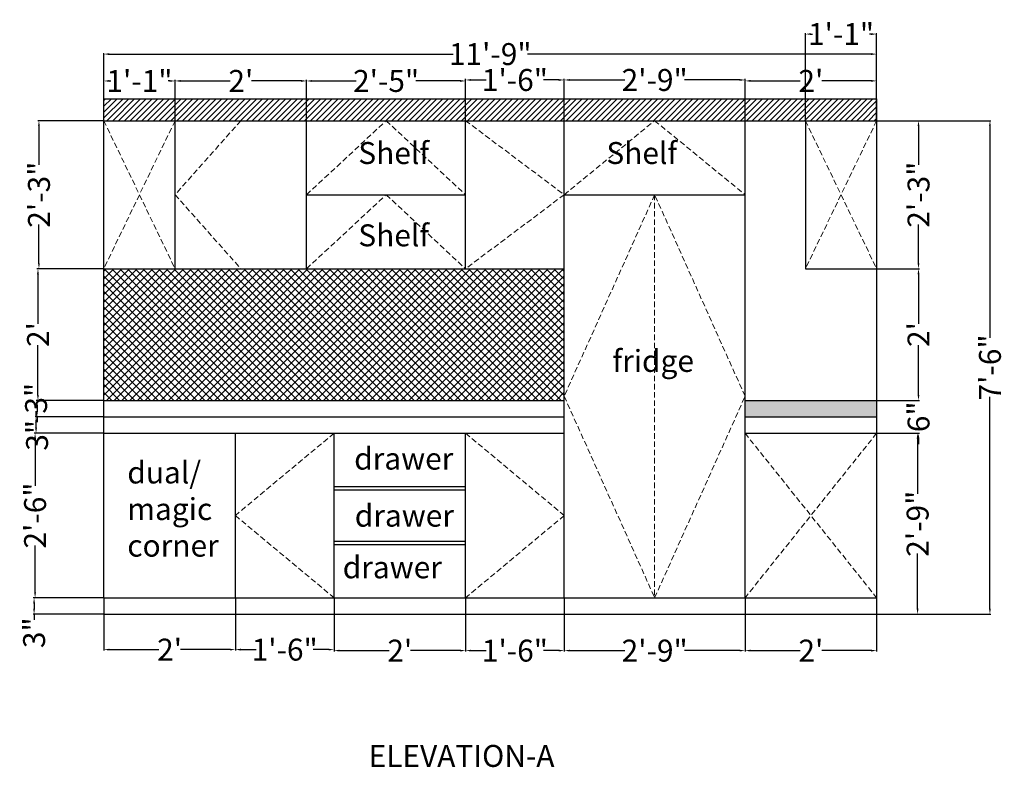
# Model space of a CAD drawing. Units: inches. Extents: x 560 to 756, y 301 to 635.
# Tile 1 of 2: x 560 to 740, y 301 to 437. Entities that reach past the tile are written whole.
import ezdxf

# ---------------------------------------------------------------- set-up
doc = ezdxf.new("R2010")
doc.units = ezdxf.units.IN
doc.header["$LTSCALE"] = 2
doc.header["$MEASUREMENT"] = 0
doc.linetypes.add('DASHED', pattern=[0.75, 0.5, -0.25])
for name, color, linetype, lineweight in [('A-ANNO-DIMS', 2, 'Continuous', 18), ('A-ANNO-TEXT', 3, 'Continuous', 18), ('A-ELEV', 7, 'Continuous', 25), ('A-ELEV-OPEN', 8, 'DASHED', 13), ('A-ELEV-PATT', 250, 'Continuous', 13)]:
    doc.layers.add(name, color=color, linetype=linetype, lineweight=lineweight)
doc.styles.get("Standard").update_dxf_attribs({"font": 'arial.ttf'})
doc.dimstyles.get("Standard").update_dxf_attribs({"dimtxt": 4, "dimasz": 1, "dimexe": 0.18, "dimexo": 0.0625, "dimgap": 0.09, "dimtad": 0, "dimdec": 0, "dimzin": 0, "dimdsep": 46, "dimlunit": 4, "dimtxsty": 'Standard', "dimcen": 0.09, "dimadec": 0, "dimazin": 0, "dimtfac": 1, "dimtdec": 0, "dimtofl": 0, "dimtmove": 0, "dimatfit": 3, "dimfxl": 1, "dimtolj": 1, "dimtzin": 0, "dimarcsym": 0})

# ---------------------------------------------------------------- blocks, each defined once
blk = doc.blocks.new('*D14')
at = {"layer": 'A-ANNO-DIMS', "color": 0, "lineweight": -2, "transparency": 16777216}
for p, q in [((575.33, 422.99), (575.33, 431.24)), ((716.33, 422.99), (716.33, 431.24)), ((576.33, 431.06), (639.06, 431.06)), ((715.33, 431.06), (652.6, 431.06))]:
    blk.add_line(p, q, dxfattribs=at)
at = {"layer": 'A-ANNO-DIMS', "color": 0, "transparency": 16777216}
for points in [[(576.33, 431.23), (576.33, 430.89), (575.33, 431.06)], [(715.33, 431.23), (715.33, 430.89), (716.33, 431.06)]]:
    blk.add_solid(points, dxfattribs=at)
at = {"layer": 'Defpoints', "color": 0, "transparency": 16777216}
for p in [(716.33, 431.06), (575.33, 422.92), (716.33, 422.92)]:
    blk.add_point(p, dxfattribs=at)
at = {"layer": 'A-ANNO-DIMS', "color": 0, "transparency": 16777216, "insert": (645.83, 431.06), "char_height": 4, "attachment_point": 5}
blk.add_mtext('\\A1;11\'-9"', dxfattribs=at)
blk = doc.blocks.new('*D15')
at = {"layer": 'A-ANNO-DIMS', "color": 0, "lineweight": -2, "transparency": 16777216}
for p, q in [((575.27, 418.92), (563.32, 418.92)), ((563.5, 417.92), (563.5, 410.86)), ((563.5, 392.92), (563.5, 399.98)), ((575.27, 391.92), (563.32, 391.92))]:
    blk.add_line(p, q, dxfattribs=at)
at = {"layer": 'A-ANNO-DIMS', "color": 0, "transparency": 16777216}
for points in [[(563.33, 417.92), (563.66, 417.92), (563.5, 418.92)], [(563.33, 392.92), (563.66, 392.92), (563.5, 391.92)]]:
    blk.add_solid(points, dxfattribs=at)
at = {"layer": 'Defpoints', "color": 0, "transparency": 16777216}
for p in [(575.33, 418.92), (563.5, 391.92), (575.33, 391.92)]:
    blk.add_point(p, dxfattribs=at)
at = {"layer": 'A-ANNO-DIMS', "color": 0, "transparency": 16777216, "insert": (563.5, 405.42), "char_height": 4, "attachment_point": 5, "rotation": 90}
blk.add_mtext('\\A1;2\'-3"', dxfattribs=at)
blk = doc.blocks.new('*D16')
at = {"layer": 'A-ANNO-DIMS', "color": 0, "lineweight": -2, "transparency": 16777216}
for p, q in [((575.27, 391.92), (563.14, 391.92)), ((563.32, 390.92), (563.32, 381.89)), ((563.32, 368.92), (563.32, 377.96)), ((575.27, 367.92), (563.14, 367.92))]:
    blk.add_line(p, q, dxfattribs=at)
at = {"layer": 'A-ANNO-DIMS', "color": 0, "transparency": 16777216}
for points in [[(563.15, 390.92), (563.48, 390.92), (563.32, 391.92)], [(563.15, 368.92), (563.48, 368.92), (563.32, 367.92)]]:
    blk.add_solid(points, dxfattribs=at)
at = {"layer": 'Defpoints', "color": 0, "transparency": 16777216}
for p in [(575.33, 391.92), (563.32, 367.92), (575.33, 367.92)]:
    blk.add_point(p, dxfattribs=at)
at = {"layer": 'A-ANNO-DIMS', "color": 0, "transparency": 16777216, "insert": (563.32, 379.92), "char_height": 4, "attachment_point": 5, "rotation": 90}
blk.add_mtext("\\A1;2'", dxfattribs=at)
blk = doc.blocks.new('*D17')
at = {"layer": 'A-ANNO-DIMS', "color": 0, "lineweight": -2, "transparency": 16777216}
for p, q in [((575.27, 367.92), (562.97, 367.92)), ((563.15, 366.92), (563.15, 365.92)), ((575.27, 364.92), (562.97, 364.92)), ((563.15, 364.92), (563.15, 363.92))]:
    blk.add_line(p, q, dxfattribs=at)
at = {"layer": 'A-ANNO-DIMS', "color": 0, "transparency": 16777216}
for points in [[(562.98, 366.92), (563.32, 366.92), (563.15, 367.92)], [(562.98, 365.92), (563.32, 365.92), (563.15, 364.92)]]:
    blk.add_solid(points, dxfattribs=at)
at = {"layer": 'Defpoints', "color": 0, "transparency": 16777216}
for p in [(575.33, 367.92), (563.15, 364.92), (575.33, 364.92)]:
    blk.add_point(p, dxfattribs=at)
at = {"layer": 'A-ANNO-DIMS', "color": 0, "transparency": 16777216, "insert": (563.15, 361.54), "char_height": 4, "attachment_point": 5, "rotation": 90}
blk.add_mtext('\\A1;3"', dxfattribs=at)
blk = doc.blocks.new('*D18')
at = {"layer": 'A-ANNO-DIMS', "color": 0, "lineweight": -2, "transparency": 16777216}
for p, q in [((575.27, 364.92), (562.79, 364.92)), ((562.97, 364.92), (562.97, 365.92)), ((562.97, 362.92), (562.97, 363.92)), ((575.27, 361.92), (562.79, 361.92))]:
    blk.add_line(p, q, dxfattribs=at)
at = {"layer": 'A-ANNO-DIMS', "color": 0, "transparency": 16777216}
for points in [[(562.8, 363.92), (563.14, 363.92), (562.97, 364.92)], [(562.8, 362.92), (563.14, 362.92), (562.97, 361.92)]]:
    blk.add_solid(points, dxfattribs=at)
at = {"layer": 'Defpoints', "color": 0, "transparency": 16777216}
for p in [(562.97, 364.92), (575.33, 364.92), (575.33, 361.92)]:
    blk.add_point(p, dxfattribs=at)
at = {"layer": 'A-ANNO-DIMS', "color": 0, "transparency": 16777216, "insert": (562.97, 368.31), "char_height": 4, "attachment_point": 5, "rotation": 90}
blk.add_mtext('\\A1;3"', dxfattribs=at)
blk = doc.blocks.new('*D19')
at = {"layer": 'A-ANNO-DIMS', "color": 0, "lineweight": -2, "transparency": 16777216}
for p, q in [((575.27, 361.92), (562.61, 361.92)), ((562.79, 360.92), (562.79, 352.36)), ((562.79, 332.92), (562.79, 341.48)), ((575.27, 331.92), (562.61, 331.92))]:
    blk.add_line(p, q, dxfattribs=at)
at = {"layer": 'A-ANNO-DIMS', "color": 0, "transparency": 16777216}
for points in [[(562.62, 360.92), (562.96, 360.92), (562.79, 361.92)], [(562.62, 332.92), (562.96, 332.92), (562.79, 331.92)]]:
    blk.add_solid(points, dxfattribs=at)
at = {"layer": 'Defpoints', "color": 0, "transparency": 16777216}
for p in [(562.79, 361.92), (575.33, 361.92), (575.33, 331.92)]:
    blk.add_point(p, dxfattribs=at)
at = {"layer": 'A-ANNO-DIMS', "color": 0, "transparency": 16777216, "insert": (562.79, 346.92), "char_height": 4, "attachment_point": 5, "rotation": 90}
blk.add_mtext('\\A1;2\'-6"', dxfattribs=at)
blk = doc.blocks.new('*D20')
at = {"layer": 'A-ANNO-DIMS', "color": 0, "lineweight": -2, "transparency": 16777216}
for p, q in [((575.27, 331.92), (562.43, 331.92)), ((562.61, 330.92), (562.61, 329.92)), ((575.27, 328.92), (562.43, 328.92)), ((562.61, 328.92), (562.61, 327.92))]:
    blk.add_line(p, q, dxfattribs=at)
at = {"layer": 'A-ANNO-DIMS', "color": 0, "transparency": 16777216}
for points in [[(562.44, 330.92), (562.78, 330.92), (562.61, 331.92)], [(562.44, 329.92), (562.78, 329.92), (562.61, 328.92)]]:
    blk.add_solid(points, dxfattribs=at)
at = {"layer": 'Defpoints', "color": 0, "transparency": 16777216}
for p in [(575.33, 331.92), (562.61, 328.92), (575.33, 328.92)]:
    blk.add_point(p, dxfattribs=at)
at = {"layer": 'A-ANNO-DIMS', "color": 0, "transparency": 16777216, "insert": (562.61, 325.54), "char_height": 4, "attachment_point": 5, "rotation": 90}
blk.add_mtext('\\A1;3"', dxfattribs=at)
blk = doc.blocks.new('*D21')
at = {"layer": 'A-ANNO-DIMS', "color": 0, "lineweight": -2, "transparency": 16777216}
for p, q in [((575.33, 331.86), (575.33, 322.28)), ((599.33, 331.86), (599.33, 322.28)), ((576.33, 322.46), (585.37, 322.46)), ((598.33, 322.46), (589.3, 322.46))]:
    blk.add_line(p, q, dxfattribs=at)
at = {"layer": 'A-ANNO-DIMS', "color": 0, "transparency": 16777216}
for points in [[(576.33, 322.63), (576.33, 322.3), (575.33, 322.46)], [(598.33, 322.63), (598.33, 322.3), (599.33, 322.46)]]:
    blk.add_solid(points, dxfattribs=at)
at = {"layer": 'Defpoints', "color": 0, "transparency": 16777216}
for p in [(575.33, 331.92), (599.33, 331.92), (599.33, 322.46)]:
    blk.add_point(p, dxfattribs=at)
at = {"layer": 'A-ANNO-DIMS', "color": 0, "transparency": 16777216, "insert": (587.33, 322.46), "char_height": 4, "attachment_point": 5}
blk.add_mtext("\\A1;2'", dxfattribs=at)
blk = doc.blocks.new('*D22')
at = {"layer": 'A-ANNO-DIMS', "color": 0, "lineweight": -2, "transparency": 16777216}
for p, q in [((599.33, 331.86), (599.33, 322.28)), ((617.33, 331.86), (617.33, 322.28)), ((600.33, 322.46), (603.11, 322.46)), ((616.33, 322.46), (613.55, 322.46))]:
    blk.add_line(p, q, dxfattribs=at)
at = {"layer": 'A-ANNO-DIMS', "color": 0, "transparency": 16777216}
for points in [[(600.33, 322.63), (600.33, 322.3), (599.33, 322.46)], [(616.33, 322.63), (616.33, 322.3), (617.33, 322.46)]]:
    blk.add_solid(points, dxfattribs=at)
at = {"layer": 'Defpoints', "color": 0, "transparency": 16777216}
for p in [(599.33, 331.92), (617.33, 331.92), (617.33, 322.46)]:
    blk.add_point(p, dxfattribs=at)
at = {"layer": 'A-ANNO-DIMS', "color": 0, "transparency": 16777216, "insert": (608.33, 322.46), "char_height": 4, "attachment_point": 5}
blk.add_mtext('\\A1;1\'-6"', dxfattribs=at)
blk = doc.blocks.new('*D23')
at = {"layer": 'A-ANNO-DIMS', "color": 0, "lineweight": -2, "transparency": 16777216}
for p, q in [((617.33, 331.86), (617.33, 322.1)), ((641.33, 331.86), (641.33, 322.1)), ((618.33, 322.28), (627.37, 322.28)), ((640.33, 322.28), (631.3, 322.28))]:
    blk.add_line(p, q, dxfattribs=at)
at = {"layer": 'A-ANNO-DIMS', "color": 0, "transparency": 16777216}
for points in [[(618.33, 322.45), (618.33, 322.12), (617.33, 322.28)], [(640.33, 322.45), (640.33, 322.12), (641.33, 322.28)]]:
    blk.add_solid(points, dxfattribs=at)
at = {"layer": 'Defpoints', "color": 0, "transparency": 16777216}
for p in [(617.33, 331.92), (641.33, 331.92), (641.33, 322.28)]:
    blk.add_point(p, dxfattribs=at)
at = {"layer": 'A-ANNO-DIMS', "color": 0, "transparency": 16777216, "insert": (629.33, 322.28), "char_height": 4, "attachment_point": 5}
blk.add_mtext("\\A1;2'", dxfattribs=at)
blk = doc.blocks.new('*D24')
at = {"layer": 'A-ANNO-DIMS', "color": 0, "lineweight": -2, "transparency": 16777216}
for p, q in [((641.33, 331.86), (641.33, 322.1)), ((659.33, 331.86), (659.33, 322.1)), ((642.33, 322.28), (645.11, 322.28)), ((658.33, 322.28), (655.55, 322.28))]:
    blk.add_line(p, q, dxfattribs=at)
at = {"layer": 'A-ANNO-DIMS', "color": 0, "transparency": 16777216}
for points in [[(642.33, 322.45), (642.33, 322.12), (641.33, 322.28)], [(658.33, 322.45), (658.33, 322.12), (659.33, 322.28)]]:
    blk.add_solid(points, dxfattribs=at)
at = {"layer": 'Defpoints', "color": 0, "transparency": 16777216}
for p in [(641.33, 331.92), (659.33, 331.92), (659.33, 322.28)]:
    blk.add_point(p, dxfattribs=at)
at = {"layer": 'A-ANNO-DIMS', "color": 0, "transparency": 16777216, "insert": (650.33, 322.28), "char_height": 4, "attachment_point": 5}
blk.add_mtext('\\A1;1\'-6"', dxfattribs=at)
blk = doc.blocks.new('*D25')
at = {"layer": 'A-ANNO-DIMS', "color": 0, "lineweight": -2, "transparency": 16777216}
for p, q in [((659.33, 331.86), (659.33, 322.1)), ((692.33, 331.86), (692.33, 322.1)), ((660.33, 322.28), (670.39, 322.28)), ((691.33, 322.28), (681.27, 322.28))]:
    blk.add_line(p, q, dxfattribs=at)
at = {"layer": 'A-ANNO-DIMS', "color": 0, "transparency": 16777216}
for points in [[(660.33, 322.45), (660.33, 322.12), (659.33, 322.28)], [(691.33, 322.45), (691.33, 322.12), (692.33, 322.28)]]:
    blk.add_solid(points, dxfattribs=at)
at = {"layer": 'Defpoints', "color": 0, "transparency": 16777216}
for p in [(659.33, 331.92), (692.33, 331.92), (692.33, 322.28)]:
    blk.add_point(p, dxfattribs=at)
at = {"layer": 'A-ANNO-DIMS', "color": 0, "transparency": 16777216, "insert": (675.83, 322.28), "char_height": 4, "attachment_point": 5}
blk.add_mtext('\\A1;2\'-9"', dxfattribs=at)
blk = doc.blocks.new('*D26')
at = {"layer": 'A-ANNO-DIMS', "color": 0, "lineweight": -2, "transparency": 16777216}
for p, q in [((692.33, 331.86), (692.33, 322.1)), ((716.33, 331.86), (716.33, 322.1)), ((693.33, 322.28), (702.37, 322.28)), ((715.33, 322.28), (706.3, 322.28))]:
    blk.add_line(p, q, dxfattribs=at)
at = {"layer": 'A-ANNO-DIMS', "color": 0, "transparency": 16777216}
for points in [[(693.33, 322.45), (693.33, 322.12), (692.33, 322.28)], [(715.33, 322.45), (715.33, 322.12), (716.33, 322.28)]]:
    blk.add_solid(points, dxfattribs=at)
at = {"layer": 'Defpoints', "color": 0, "transparency": 16777216}
for p in [(692.33, 331.92), (716.33, 331.92), (716.33, 322.28)]:
    blk.add_point(p, dxfattribs=at)
at = {"layer": 'A-ANNO-DIMS', "color": 0, "transparency": 16777216, "insert": (704.33, 322.28), "char_height": 4, "attachment_point": 5}
blk.add_mtext("\\A1;2'", dxfattribs=at)
blk = doc.blocks.new('*D27')
at = {"layer": 'A-ANNO-DIMS', "color": 0, "lineweight": -2, "transparency": 16777216}
for p, q in [((716.39, 418.92), (737.18, 418.92)), ((737, 417.92), (737, 379.31)), ((737, 329.92), (737, 368.53)), ((716.39, 328.92), (737.18, 328.92))]:
    blk.add_line(p, q, dxfattribs=at)
at = {"layer": 'A-ANNO-DIMS', "color": 0, "transparency": 16777216}
for points in [[(736.83, 417.92), (737.16, 417.92), (737, 418.92)], [(736.83, 329.92), (737.16, 329.92), (737, 328.92)]]:
    blk.add_solid(points, dxfattribs=at)
at = {"layer": 'Defpoints', "color": 0, "transparency": 16777216}
for p in [(716.33, 418.92), (716.33, 328.92), (737, 328.92)]:
    blk.add_point(p, dxfattribs=at)
at = {"layer": 'A-ANNO-DIMS', "color": 0, "transparency": 16777216, "insert": (737, 373.92), "char_height": 4, "attachment_point": 5, "rotation": 90}
blk.add_mtext('\\A1;7\'-6"', dxfattribs=at)
blk = doc.blocks.new('*D28')
at = {"layer": 'A-ANNO-DIMS', "color": 0, "lineweight": -2, "transparency": 16777216}
for p, q in [((575.33, 418.99), (575.33, 426.34)), ((576.33, 426.16), (576.61, 426.16)), ((587.33, 426.16), (587.05, 426.16)), ((588.33, 418.99), (588.33, 426.34))]:
    blk.add_line(p, q, dxfattribs=at)
at = {"layer": 'A-ANNO-DIMS', "color": 0, "transparency": 16777216}
for points in [[(576.33, 426.33), (576.33, 425.99), (575.33, 426.16)], [(587.33, 426.33), (587.33, 425.99), (588.33, 426.16)]]:
    blk.add_solid(points, dxfattribs=at)
at = {"layer": 'Defpoints', "color": 0, "transparency": 16777216}
for p in [(588.33, 426.16), (575.33, 418.92), (588.33, 418.92)]:
    blk.add_point(p, dxfattribs=at)
at = {"layer": 'A-ANNO-DIMS', "color": 0, "transparency": 16777216, "insert": (581.83, 426.16), "char_height": 4, "attachment_point": 5}
blk.add_mtext('\\A1;1\'-1"', dxfattribs=at)
blk = doc.blocks.new('*D29')
at = {"layer": 'A-ANNO-DIMS', "color": 0, "lineweight": -2, "transparency": 16777216}
for p, q in [((588.33, 418.99), (588.33, 426.34)), ((589.33, 426.16), (598.37, 426.16)), ((611.33, 426.16), (602.3, 426.16)), ((612.33, 418.99), (612.33, 426.34))]:
    blk.add_line(p, q, dxfattribs=at)
at = {"layer": 'A-ANNO-DIMS', "color": 0, "transparency": 16777216}
for points in [[(589.33, 426.33), (589.33, 425.99), (588.33, 426.16)], [(611.33, 426.33), (611.33, 425.99), (612.33, 426.16)]]:
    blk.add_solid(points, dxfattribs=at)
at = {"layer": 'Defpoints', "color": 0, "transparency": 16777216}
for p in [(612.33, 426.16), (588.33, 418.92), (612.33, 418.92)]:
    blk.add_point(p, dxfattribs=at)
at = {"layer": 'A-ANNO-DIMS', "color": 0, "transparency": 16777216, "insert": (600.33, 426.16), "char_height": 4, "attachment_point": 5}
blk.add_mtext("\\A1;2'", dxfattribs=at)
blk = doc.blocks.new('*D30')
at = {"layer": 'A-ANNO-DIMS', "color": 0, "lineweight": -2, "transparency": 16777216}
for p, q in [((612.33, 418.99), (612.33, 426.34)), ((613.33, 426.16), (621.39, 426.16)), ((640.33, 426.16), (632.27, 426.16)), ((641.33, 418.99), (641.33, 426.34))]:
    blk.add_line(p, q, dxfattribs=at)
at = {"layer": 'A-ANNO-DIMS', "color": 0, "transparency": 16777216}
for points in [[(613.33, 426.33), (613.33, 425.99), (612.33, 426.16)], [(640.33, 426.33), (640.33, 425.99), (641.33, 426.16)]]:
    blk.add_solid(points, dxfattribs=at)
at = {"layer": 'Defpoints', "color": 0, "transparency": 16777216}
for p in [(641.33, 426.16), (612.33, 418.92), (641.33, 418.92)]:
    blk.add_point(p, dxfattribs=at)
at = {"layer": 'A-ANNO-DIMS', "color": 0, "transparency": 16777216, "insert": (626.83, 426.16), "char_height": 4, "attachment_point": 5}
blk.add_mtext('\\A1;2\'-5"', dxfattribs=at)
blk = doc.blocks.new('*D31')
at = {"layer": 'A-ANNO-DIMS', "color": 0, "lineweight": -2, "transparency": 16777216}
for p, q in [((641.33, 418.99), (641.33, 426.52)), ((642.33, 426.34), (645.11, 426.34)), ((658.33, 426.34), (655.55, 426.34)), ((659.33, 418.99), (659.33, 426.52))]:
    blk.add_line(p, q, dxfattribs=at)
at = {"layer": 'A-ANNO-DIMS', "color": 0, "transparency": 16777216}
for points in [[(642.33, 426.51), (642.33, 426.17), (641.33, 426.34)], [(658.33, 426.51), (658.33, 426.17), (659.33, 426.34)]]:
    blk.add_solid(points, dxfattribs=at)
at = {"layer": 'Defpoints', "color": 0, "transparency": 16777216}
for p in [(659.33, 426.34), (641.33, 418.92), (659.33, 418.92)]:
    blk.add_point(p, dxfattribs=at)
at = {"layer": 'A-ANNO-DIMS', "color": 0, "transparency": 16777216, "insert": (650.33, 426.34), "char_height": 4, "attachment_point": 5}
blk.add_mtext('\\A1;1\'-6"', dxfattribs=at)
blk = doc.blocks.new('*D32')
at = {"layer": 'A-ANNO-DIMS', "color": 0, "lineweight": -2, "transparency": 16777216}
for p, q in [((659.33, 418.99), (659.33, 426.52)), ((660.33, 426.34), (670.39, 426.34)), ((691.33, 426.34), (681.27, 426.34)), ((692.33, 418.99), (692.33, 426.52))]:
    blk.add_line(p, q, dxfattribs=at)
at = {"layer": 'A-ANNO-DIMS', "color": 0, "transparency": 16777216}
for points in [[(660.33, 426.51), (660.33, 426.17), (659.33, 426.34)], [(691.33, 426.51), (691.33, 426.17), (692.33, 426.34)]]:
    blk.add_solid(points, dxfattribs=at)
at = {"layer": 'Defpoints', "color": 0, "transparency": 16777216}
for p in [(692.33, 426.34), (659.33, 418.92), (692.33, 418.92)]:
    blk.add_point(p, dxfattribs=at)
at = {"layer": 'A-ANNO-DIMS', "color": 0, "transparency": 16777216, "insert": (675.83, 426.34), "char_height": 4, "attachment_point": 5}
blk.add_mtext('\\A1;2\'-9"', dxfattribs=at)
blk = doc.blocks.new('*D33')
at = {"layer": 'A-ANNO-DIMS', "color": 0, "lineweight": -2, "transparency": 16777216}
for p, q in [((692.33, 418.99), (692.33, 426.35)), ((693.33, 426.17), (702.37, 426.17)), ((715.33, 426.17), (706.3, 426.17)), ((716.33, 418.99), (716.33, 426.35))]:
    blk.add_line(p, q, dxfattribs=at)
at = {"layer": 'A-ANNO-DIMS', "color": 0, "transparency": 16777216}
for points in [[(693.33, 426.34), (693.33, 426.01), (692.33, 426.17)], [(715.33, 426.34), (715.33, 426.01), (716.33, 426.17)]]:
    blk.add_solid(points, dxfattribs=at)
at = {"layer": 'Defpoints', "color": 0, "transparency": 16777216}
for p in [(716.33, 426.17), (692.33, 418.92), (716.33, 418.92)]:
    blk.add_point(p, dxfattribs=at)
at = {"layer": 'A-ANNO-DIMS', "color": 0, "transparency": 16777216, "insert": (704.33, 426.17), "char_height": 4, "attachment_point": 5}
blk.add_mtext("\\A1;2'", dxfattribs=at)
blk = doc.blocks.new('*D34')
at = {"layer": 'A-ANNO-DIMS', "color": 0, "lineweight": -2, "transparency": 16777216}
for p, q in [((703.33, 418.99), (703.33, 434.89)), ((716.33, 418.99), (716.33, 434.89)), ((704.33, 434.71), (704.61, 434.71)), ((715.33, 434.71), (715.05, 434.71))]:
    blk.add_line(p, q, dxfattribs=at)
at = {"layer": 'A-ANNO-DIMS', "color": 0, "transparency": 16777216}
for points in [[(704.33, 434.87), (704.33, 434.54), (703.33, 434.71)], [(715.33, 434.87), (715.33, 434.54), (716.33, 434.71)]]:
    blk.add_solid(points, dxfattribs=at)
at = {"layer": 'Defpoints', "color": 0, "transparency": 16777216}
for p in [(716.33, 434.71), (703.33, 418.92), (716.33, 418.92)]:
    blk.add_point(p, dxfattribs=at)
at = {"layer": 'A-ANNO-DIMS', "color": 0, "transparency": 16777216, "insert": (709.83, 434.71), "char_height": 4, "attachment_point": 5}
blk.add_mtext('\\A1;1\'-1"', dxfattribs=at)
blk = doc.blocks.new('*D35')
at = {"layer": 'A-ANNO-DIMS', "color": 0, "lineweight": -2, "transparency": 16777216}
for p, q in [((716.39, 418.92), (724.15, 418.92)), ((723.97, 417.92), (723.97, 410.86)), ((723.97, 392.92), (723.97, 399.98)), ((716.39, 391.92), (724.15, 391.92))]:
    blk.add_line(p, q, dxfattribs=at)
at = {"layer": 'A-ANNO-DIMS', "color": 0, "transparency": 16777216}
for points in [[(723.8, 417.92), (724.13, 417.92), (723.97, 418.92)], [(723.8, 392.92), (724.13, 392.92), (723.97, 391.92)]]:
    blk.add_solid(points, dxfattribs=at)
at = {"layer": 'Defpoints', "color": 0, "transparency": 16777216}
for p in [(716.33, 418.92), (716.33, 391.92), (723.97, 391.92)]:
    blk.add_point(p, dxfattribs=at)
at = {"layer": 'A-ANNO-DIMS', "color": 0, "transparency": 16777216, "insert": (723.97, 405.42), "char_height": 4, "attachment_point": 5, "rotation": 90}
blk.add_mtext('\\A1;2\'-3"', dxfattribs=at)
blk = doc.blocks.new('*D36')
at = {"layer": 'A-ANNO-DIMS', "color": 0, "lineweight": -2, "transparency": 16777216}
for p, q in [((716.39, 391.92), (724.15, 391.92)), ((723.97, 390.92), (723.97, 381.89)), ((723.97, 368.92), (723.97, 377.96)), ((716.39, 367.92), (724.15, 367.92))]:
    blk.add_line(p, q, dxfattribs=at)
at = {"layer": 'A-ANNO-DIMS', "color": 0, "transparency": 16777216}
for points in [[(723.8, 390.92), (724.13, 390.92), (723.97, 391.92)], [(723.8, 368.92), (724.13, 368.92), (723.97, 367.92)]]:
    blk.add_solid(points, dxfattribs=at)
at = {"layer": 'Defpoints', "color": 0, "transparency": 16777216}
for p in [(716.33, 391.92), (716.33, 367.92), (723.97, 367.92)]:
    blk.add_point(p, dxfattribs=at)
at = {"layer": 'A-ANNO-DIMS', "color": 0, "transparency": 16777216, "insert": (723.97, 379.92), "char_height": 4, "attachment_point": 5, "rotation": 90}
blk.add_mtext("\\A1;2'", dxfattribs=at)
blk = doc.blocks.new('*D37')
at = {"layer": 'A-ANNO-DIMS', "color": 0, "lineweight": -2, "transparency": 16777216}
for p, q in [((723.97, 368.92), (723.97, 369.92)), ((716.39, 367.92), (724.15, 367.92)), ((716.39, 361.92), (724.15, 361.92)), ((723.97, 360.92), (723.97, 359.92))]:
    blk.add_line(p, q, dxfattribs=at)
at = {"layer": 'A-ANNO-DIMS', "color": 0, "transparency": 16777216}
for points in [[(723.8, 368.92), (724.13, 368.92), (723.97, 367.92)], [(723.8, 360.92), (724.13, 360.92), (723.97, 361.92)]]:
    blk.add_solid(points, dxfattribs=at)
at = {"layer": 'Defpoints', "color": 0, "transparency": 16777216}
for p in [(716.33, 367.92), (716.33, 361.92), (723.97, 361.92)]:
    blk.add_point(p, dxfattribs=at)
at = {"layer": 'A-ANNO-DIMS', "color": 0, "transparency": 16777216, "insert": (723.97, 364.92), "char_height": 4, "attachment_point": 5, "rotation": 90}
blk.add_mtext('\\A1;6"', dxfattribs=at)
blk = doc.blocks.new('*D38')
at = {"layer": 'A-ANNO-DIMS', "color": 0, "lineweight": -2, "transparency": 16777216}
for p, q in [((716.39, 361.92), (723.98, 361.92)), ((723.8, 360.92), (723.8, 350.86)), ((723.8, 329.92), (723.8, 339.98)), ((716.39, 328.92), (723.98, 328.92))]:
    blk.add_line(p, q, dxfattribs=at)
at = {"layer": 'A-ANNO-DIMS', "color": 0, "transparency": 16777216}
for points in [[(723.63, 360.92), (723.97, 360.92), (723.8, 361.92)], [(723.63, 329.92), (723.97, 329.92), (723.8, 328.92)]]:
    blk.add_solid(points, dxfattribs=at)
at = {"layer": 'Defpoints', "color": 0, "transparency": 16777216}
for p in [(716.33, 361.92), (716.33, 328.92), (723.8, 328.92)]:
    blk.add_point(p, dxfattribs=at)
at = {"layer": 'A-ANNO-DIMS', "color": 0, "transparency": 16777216, "insert": (723.8, 345.42), "char_height": 4, "attachment_point": 5, "rotation": 90}
blk.add_mtext('\\A1;2\'-9"', dxfattribs=at)

msp = doc.modelspace()

# ---------------------------------------------------------------- hatches: boundary and pattern name
at = {"layer": 'A-ELEV-PATT'}
h = msp.add_hatch(dxfattribs=at)
h.set_pattern_fill('ANSI31', color=256, scale=6)
h.paths.add_polyline_path([(716.33, 422.92), (575.33, 422.92), (575.33, 418.92), (716.33, 418.92)])
h = msp.add_hatch(dxfattribs=at)
h.set_pattern_fill('ANSI37', color=256, scale=8)
h.paths.add_polyline_path([(659.33, 391.92), (575.33, 391.92), (575.33, 367.92), (659.33, 367.92)])
h = msp.add_hatch(color=256, dxfattribs=at)
h.dxf.hatch_style = 1
h.paths.add_polyline_path([(716.33, 367.92), (692.33, 367.92), (692.33, 364.92), (716.33, 364.92)])

# ---------------------------------------------------------------- linework, layer by layer
at = {"layer": 'A-ELEV'}
for p, q in [((575.33, 418.92), (575.33, 422.92)), ((575.33, 422.92), (716.33, 422.92)), ((716.33, 422.92), (716.33, 418.92)), ((575.33, 418.92), (716.33, 418.92)), ((575.33, 361.92), (575.33, 418.92)), ((588.33, 391.92), (588.33, 418.92)), ((612.33, 391.92), (612.33, 418.92)), ((641.33, 391.92), (641.33, 418.92)), ((659.33, 331.92), (659.33, 418.92)), ((692.33, 331.92), (692.33, 418.92)), ((703.33, 418.92), (703.33, 391.92)), ((716.33, 418.92), (716.33, 328.92)), ((612.33, 405.42), (641.33, 405.42)), ((659.33, 405.42), (692.33, 405.42)), ((575.33, 391.92), (659.33, 391.92)), ((703.33, 391.92), (716.33, 391.92)), ((575.33, 367.92), (659.33, 367.92)), ((692.33, 367.92), (716.33, 367.92)), ((575.33, 364.92), (659.33, 364.92)), ((692.33, 364.92), (716.33, 364.92)), ((575.33, 331.92), (575.33, 361.92)), ((575.33, 361.92), (659.33, 361.92)), ((599.33, 331.92), (599.33, 361.92)), ((617.33, 331.92), (617.33, 361.92)), ((641.33, 331.92), (641.33, 361.92)), ((692.33, 361.92), (716.33, 361.92)), ((617.33, 352.22), (641.33, 352.22)), ((617.33, 351.62), (641.33, 351.62)), ((617.33, 342.22), (641.33, 342.22)), ((617.33, 341.62), (641.33, 341.62)), ((575.33, 331.92), (659.33, 331.92)), ((575.33, 331.92), (575.33, 328.92)), ((659.33, 331.92), (716.33, 331.92)), ((575.33, 328.92), (716.33, 328.92))]:
    msp.add_line(p, q, dxfattribs=at)
at = {"layer": 'A-ELEV-OPEN'}
for p, q in [((575.33, 418.92), (588.33, 391.92)), ((588.33, 418.92), (575.33, 391.92)), ((600.33, 418.92), (588.33, 405.42)), ((612.33, 405.42), (626.83, 418.92)), ((626.83, 418.92), (641.33, 405.42)), ((641.33, 418.92), (659.33, 405.42)), ((659.33, 405.42), (675.83, 418.92)), ((675.83, 418.92), (692.33, 405.42)), ((703.33, 418.92), (716.33, 391.92)), ((716.33, 418.92), (703.33, 391.92)), ((588.33, 405.42), (600.33, 391.92)), ((612.33, 391.92), (626.83, 405.42)), ((626.83, 405.42), (641.33, 391.92)), ((659.33, 405.42), (641.33, 391.92)), ((675.83, 405.42), (659.33, 368.67)), ((692.33, 368.67), (675.83, 405.42)), ((675.83, 405.42), (675.83, 331.92)), ((659.33, 368.67), (675.83, 331.92)), ((675.83, 331.92), (692.33, 368.67)), ((617.33, 361.92), (599.33, 346.92)), ((641.33, 361.92), (659.33, 346.92)), ((692.33, 361.92), (716.33, 331.92)), ((716.33, 361.92), (692.33, 331.92)), ((599.33, 346.92), (617.33, 331.92)), ((659.33, 346.92), (641.33, 331.92))]:
    msp.add_line(p, q, dxfattribs=at)

# ---------------------------------------------------------------- texts
at = {"layer": 'A-ANNO-TEXT', "char_height": 4, "attachment_point": 1}
for s, width, heights, insert in [('\\pxqc;Shelf', 26.2343, [0], (615.1, 415.02)), ('\\pxqc;Shelf', 26.2343, [0], (660.36, 415.02)), ('\\pxqc;Shelf', 26.2343, [0], (615.1, 400.01)), ('\\pxqc;fridge', 21.761, [0], (664.69, 377.11)), ('drawer', 21.4632, [0], (621.01, 359.29)), ('dual/\\Pmagic corner', 19.4622, [0], (579.62, 356.76)), ('drawer', 21.4632, [0], (621.12, 348.89)), ('drawer', 21.4632, [0], (618.92, 339.47)), ('\\pxqc;ELEVATION-A', 88.5047, [4], (596.34, 305.08))]:
    msp.add_mtext_dynamic_manual_height_columns(s, width=width, gutter_width=20, heights=heights, dxfattribs=dict(at, insert=insert))

# ---------------------------------------------------------------- dimensions: what is measured, and where the dimension line sits
at = {"layer": 'A-ANNO-DIMS'}
for base, p1, p2, picture, middle in [((716.33, 434.71), (703.33, 418.92), (716.33, 418.92), '*D34', (709.83, 434.71)), ((716.33, 431.06), (575.33, 422.92), (716.33, 422.92), '*D14', (645.83, 431.06)), ((588.33, 426.16), (575.33, 418.92), (588.33, 418.92), '*D28', (581.83, 426.16)), ((612.33, 426.16), (588.33, 418.92), (612.33, 418.92), '*D29', (600.33, 426.16)), ((641.33, 426.16), (612.33, 418.92), (641.33, 418.92), '*D30', (626.83, 426.16)), ((659.33, 426.34), (641.33, 418.92), (659.33, 418.92), '*D31', (650.33, 426.34)), ((692.33, 426.34), (659.33, 418.92), (692.33, 418.92), '*D32', (675.83, 426.34)), ((716.33, 426.17), (692.33, 418.92), (716.33, 418.92), '*D33', (704.33, 426.17)), ((599.33, 322.46), (575.33, 331.92), (599.33, 331.92), '*D21', (587.33, 322.46)), ((617.33, 322.46), (599.33, 331.92), (617.33, 331.92), '*D22', (608.33, 322.46)), ((641.33, 322.28), (617.33, 331.92), (641.33, 331.92), '*D23', (629.33, 322.28)), ((659.33, 322.28), (641.33, 331.92), (659.33, 331.92), '*D24', (650.33, 322.28)), ((692.33, 322.28), (659.33, 331.92), (692.33, 331.92), '*D25', (675.83, 322.28)), ((716.33, 322.28), (692.33, 331.92), (716.33, 331.92), '*D26', (704.33, 322.28))]:
    dim = msp.add_linear_dim(base=base, p1=p1, p2=p2, dimstyle='Standard', override={"dimclrd": 0, "dimclre": 0, "dimclrt": 0}, dxfattribs=at)
    dim.commit()
    dim.dimension.update_dxf_attribs({"geometry": picture, "text_midpoint": middle})
for base, p1, p2, picture, middle in [((563.5, 391.92), (575.33, 418.92), (575.33, 391.92), '*D15', (563.5, 405.42)), ((737, 328.92), (716.33, 418.92), (716.33, 328.92), '*D27', (737, 373.92)), ((723.97, 391.92), (716.33, 418.92), (716.33, 391.92), '*D35', (723.97, 405.42)), ((563.32, 367.92), (575.33, 391.92), (575.33, 367.92), '*D16', (563.32, 379.92)), ((723.97, 367.92), (716.33, 391.92), (716.33, 367.92), '*D36', (723.97, 379.92)), ((562.97, 364.92), (575.33, 361.92), (575.33, 364.92), '*D18', (562.97, 368.31)), ((723.97, 361.92), (716.33, 367.92), (716.33, 361.92), '*D37', (723.97, 364.92)), ((563.15, 364.92), (575.33, 367.92), (575.33, 364.92), '*D17', (563.15, 361.54)), ((562.79, 361.92), (575.33, 331.92), (575.33, 361.92), '*D19', (562.79, 346.92)), ((723.8, 328.92), (716.33, 361.92), (716.33, 328.92), '*D38', (723.8, 345.42)), ((562.61, 328.92), (575.33, 331.92), (575.33, 328.92), '*D20', (562.61, 325.54))]:
    dim = msp.add_linear_dim(base=base, p1=p1, p2=p2, angle=90, dimstyle='Standard', override={"dimclrd": 0, "dimclre": 0, "dimclrt": 0}, dxfattribs=at)
    dim.commit()
    dim.dimension.update_dxf_attribs({"geometry": picture, "text_midpoint": middle})

doc.saveas('drawing.dxf')
